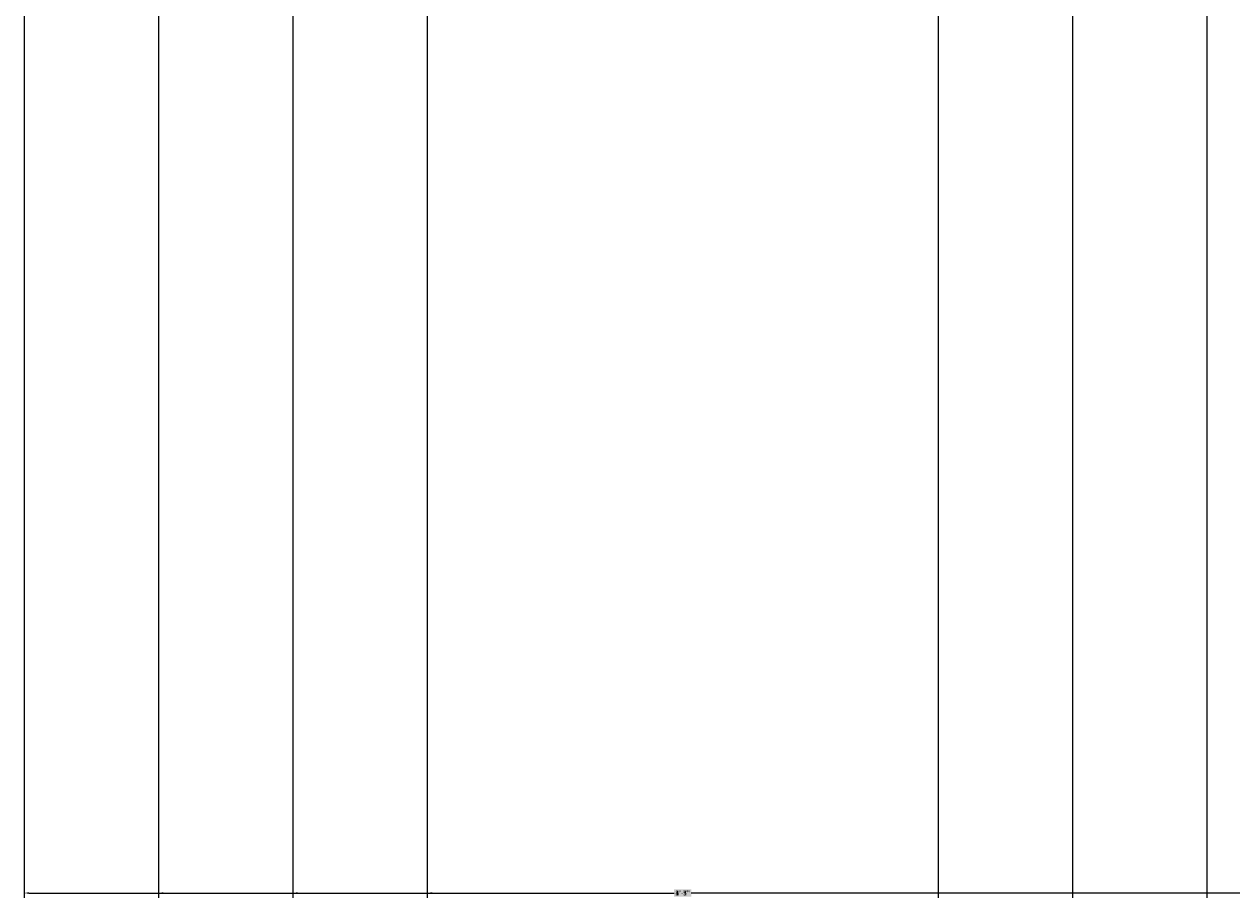
# Model space of a CAD drawing. Units: inches. Extents: x -301 to 715, y -607 to 364.
# Tile 27 of 141: x 114 to 159, y -574 to -541. Entities that reach past the tile are written whole.
import ezdxf

# ---------------------------------------------------------------- set-up
doc = ezdxf.new("R2010")
doc.units = ezdxf.units.IN
doc.header["$MEASUREMENT"] = 0
doc.layers.add('A-ANNO-DIMS', color=2, linetype='Continuous', lineweight=18)
doc.styles.get("Standard").update_dxf_attribs({"font": 'arial.ttf'})
doc.dimstyles.get("Standard").update_dxf_attribs({"dimtxt": 0.18, "dimasz": 0.18, "dimexe": 0.18, "dimexo": 0.0625, "dimgap": 0.09, "dimtad": 0, "dimtih": 1, "dimtoh": 1, "dimdec": 1, "dimzin": 0, "dimdsep": 46, "dimlunit": 4, "dimtxsty": 'Standard', "dimcen": 0.09, "dimclrd": 3, "dimclre": 4, "dimclrt": 6, "dimadec": 0, "dimazin": 0, "dimtfac": 1, "dimtdec": 1, "dimtofl": 0, "dimtmove": 0, "dimatfit": 3, "dimfxl": 1, "dimtfill": 2, "dimtfillclr": 51, "dimtolj": 1, "dimtzin": 0, "dimarcsym": 0})

# ---------------------------------------------------------------- blocks, each defined once
blk = doc.blocks.new('*D182')
at = {"layer": 'A-ANNO-DIMS', "color": 4, "lineweight": -2, "transparency": 16777216}
for p, q in [((114.255, -540.54), (114.255, -573.809)), ((163.255, -540.54), (163.255, -573.809))]:
    blk.add_line(p, q, dxfattribs=at)
at = {"layer": 'A-ANNO-DIMS', "color": 3, "lineweight": -2, "transparency": 16777216}
for p, q in [((114.435, -573.629), (138.422, -573.629)), ((163.075, -573.629), (139.088, -573.629))]:
    blk.add_line(p, q, dxfattribs=at)
at = {"layer": 'A-ANNO-DIMS', "color": 3, "transparency": 16777216}
for points in [[(114.435, -573.599), (114.435, -573.659), (114.255, -573.629)], [(163.075, -573.599), (163.075, -573.659), (163.255, -573.629)]]:
    blk.add_solid(points, dxfattribs=at)
at = {"layer": 'Defpoints', "color": 0, "transparency": 16777216}
for p in [(114.255, -540.477), (163.255, -540.477), (163.255, -573.629)]:
    blk.add_point(p, dxfattribs=at)
at = {"layer": 'A-ANNO-DIMS', "color": 6, "transparency": 16777216, "insert": (138.755, -573.629), "char_height": 0.18, "attachment_point": 5, "bg_fill": 1, "box_fill_scale": 1.25, "bg_fill_color": 51, "bg_fill_transparency": 0}
blk.add_mtext('\\A1;4\'-1"', dxfattribs=at)
blk = doc.blocks.new('*D183')
at = {"layer": 'A-ANNO-DIMS', "color": 4, "lineweight": -2, "transparency": 16777216}
for p, q in [((119.255, -535.54), (119.255, -573.809)), ((158.255, -535.54), (158.255, -573.809))]:
    blk.add_line(p, q, dxfattribs=at)
at = {"layer": 'A-ANNO-DIMS', "color": 3, "lineweight": -2, "transparency": 16777216}
for p, q in [((119.435, -573.629), (138.426, -573.629)), ((158.075, -573.629), (139.084, -573.629))]:
    blk.add_line(p, q, dxfattribs=at)
at = {"layer": 'A-ANNO-DIMS', "color": 3, "transparency": 16777216}
for points in [[(119.435, -573.599), (119.435, -573.659), (119.255, -573.629)], [(158.075, -573.599), (158.075, -573.659), (158.255, -573.629)]]:
    blk.add_solid(points, dxfattribs=at)
at = {"layer": 'Defpoints', "color": 0, "transparency": 16777216}
for p in [(119.255, -535.477), (158.255, -535.477), (158.255, -573.629)]:
    blk.add_point(p, dxfattribs=at)
at = {"layer": 'A-ANNO-DIMS', "color": 6, "transparency": 16777216, "insert": (138.755, -573.629), "char_height": 0.18, "attachment_point": 5, "bg_fill": 1, "box_fill_scale": 1.25, "bg_fill_color": 51, "bg_fill_transparency": 0}
blk.add_mtext('\\A1;3\'-3"', dxfattribs=at)
blk = doc.blocks.new('*D184')
at = {"layer": 'A-ANNO-DIMS', "color": 4, "lineweight": -2, "transparency": 16777216}
for p, q in [((124.255, -511.54), (124.255, -573.809)), ((153.255, -511.54), (153.255, -573.809))]:
    blk.add_line(p, q, dxfattribs=at)
at = {"layer": 'A-ANNO-DIMS', "color": 3, "lineweight": -2, "transparency": 16777216}
for p, q in [((124.435, -573.629), (138.424, -573.629)), ((153.075, -573.629), (139.086, -573.629))]:
    blk.add_line(p, q, dxfattribs=at)
at = {"layer": 'A-ANNO-DIMS', "color": 3, "transparency": 16777216}
for points in [[(124.435, -573.599), (124.435, -573.659), (124.255, -573.629)], [(153.075, -573.599), (153.075, -573.659), (153.255, -573.629)]]:
    blk.add_solid(points, dxfattribs=at)
at = {"layer": 'Defpoints', "color": 0, "transparency": 16777216}
for p in [(124.255, -511.477), (153.255, -511.477), (153.255, -573.629)]:
    blk.add_point(p, dxfattribs=at)
at = {"layer": 'A-ANNO-DIMS', "color": 6, "transparency": 16777216, "insert": (138.755, -573.629), "char_height": 0.18, "attachment_point": 5, "bg_fill": 1, "box_fill_scale": 1.25, "bg_fill_color": 51, "bg_fill_transparency": 0}
blk.add_mtext('\\A1;2\'-5"', dxfattribs=at)
blk = doc.blocks.new('*D185')
at = {"layer": 'A-ANNO-DIMS', "color": 4, "lineweight": -2, "transparency": 16777216}
for p, q in [((129.255, -493.54), (129.255, -573.809)), ((148.255, -493.54), (148.255, -573.809))]:
    blk.add_line(p, q, dxfattribs=at)
at = {"layer": 'A-ANNO-DIMS', "color": 3, "lineweight": -2, "transparency": 16777216}
for p, q in [((129.435, -573.629), (138.434, -573.629)), ((148.075, -573.629), (139.076, -573.629))]:
    blk.add_line(p, q, dxfattribs=at)
at = {"layer": 'A-ANNO-DIMS', "color": 3, "transparency": 16777216}
for points in [[(129.435, -573.599), (129.435, -573.659), (129.255, -573.629)], [(148.075, -573.599), (148.075, -573.659), (148.255, -573.629)]]:
    blk.add_solid(points, dxfattribs=at)
at = {"layer": 'Defpoints', "color": 0, "transparency": 16777216}
for p in [(129.255, -493.477), (148.255, -493.477), (148.255, -573.629)]:
    blk.add_point(p, dxfattribs=at)
at = {"layer": 'A-ANNO-DIMS', "color": 6, "transparency": 16777216, "insert": (138.755, -573.629), "char_height": 0.18, "attachment_point": 5, "bg_fill": 1, "box_fill_scale": 1.25, "bg_fill_color": 51, "bg_fill_transparency": 0}
blk.add_mtext('\\A1;1\'-7"', dxfattribs=at)

msp = doc.modelspace()

# ---------------------------------------------------------------- dimensions: what is measured, and where the dimension line sits
at = {"layer": 'A-ANNO-DIMS'}
for base, p1, p2, picture in [((148.255, -573.629), (129.255, -493.477), (148.255, -493.477), '*D185'), ((153.255, -573.629), (124.255, -511.477), (153.255, -511.477), '*D184'), ((158.255, -573.629), (119.255, -535.477), (158.255, -535.477), '*D183'), ((163.255, -573.629), (114.255, -540.477), (163.255, -540.477), '*D182')]:
    dim = msp.add_linear_dim(base=base, p1=p1, p2=p2, dimstyle='Standard', override={"dimdec": 1, "dimlfac": 1, "dimrnd": 0, "dimzin": 1, "dimdsep": 46, "dimlunit": 4, "dimfrac": 2}, dxfattribs=at)
    dim.commit()
    dim.dimension.update_dxf_attribs({"geometry": picture, "text_midpoint": (138.755, -573.629)})

doc.saveas('drawing.dxf')
